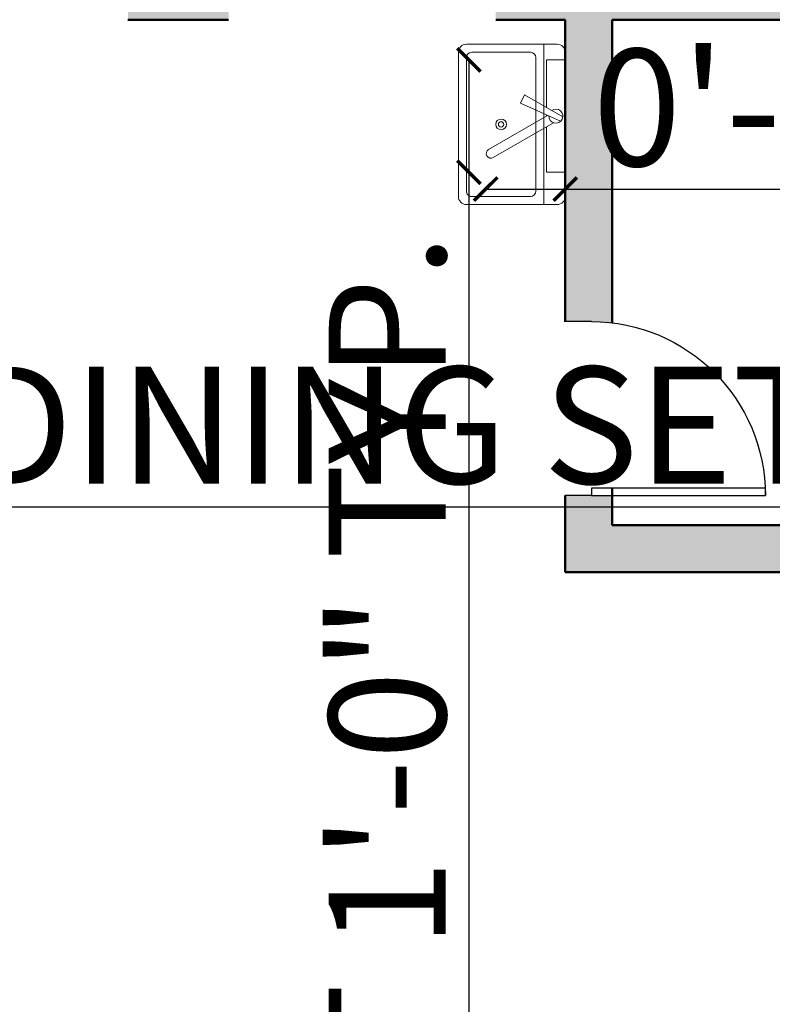
# Model space of a CAD drawing. Units: inches. Extents: x 2419 to 2878, y 1068 to 1713.
# Tile 11 of 20: x 2574 to 2655, y 1304 to 1409. Entities that reach past the tile are written whole.
import ezdxf

# ---------------------------------------------------------------- set-up
doc = ezdxf.new("R2010")
doc.units = ezdxf.units.IN
for name, color, linetype, lineweight in [('A-ANNO-DIMS', 2, 'Continuous', 18), ('A-DOOR', 4, 'Continuous', 25), ('A-FLOR-FIXT', 8, 'Continuous', 18), ('A-FLOR-PRKG-PATT', 1, 'Continuous', 13), ('A-WALL', 7, 'Continuous', 50)]:
    doc.layers.add(name, color=color, linetype=linetype, lineweight=lineweight)
doc.layers.add('A-WALL-PATT', color=18, linetype='Continuous', lineweight=13, true_color=0x000000)
doc.styles.get("Standard").update_dxf_attribs({"font": 'arial.ttf'})
doc.dimstyles.new('ISO-25', dxfattribs={"dimtxt": 12.5, "dimasz": 2.5, "dimexe": 1.25, "dimexo": 0.625, "dimtad": 1, "dimdec": 0, "dimlunit": 4, "dimtxsty": 'Standard', "dimblk": 'ARCHTICK', "dimcen": 2.5, "dimse1": 1, "dimse2": 1, "dimclrd": 4, "dimadec": 0, "dimazin": 0, "dimtfac": 1, "dimtdec": 0, "dimtmove": 0, "dimatfit": 3, "dimfxl": 1, "dimarcsym": 0})

# ---------------------------------------------------------------- blocks, each defined once
blk = doc.blocks.new('*U3')
for p, q in [((0, 0), (0, -6)), ((40, 0), (40, -6))]:
    blk.add_line(p, q)
blk.add_lwpolyline([(0, 0), (0, 40), (1.75, 40), (1.75, 0)], close=True)
blk.add_arc((0, 0), 40, 0, 90)
blk = doc.blocks.new('Sink-single - 30 in top')
blk.add_line((-15, -3.999996), (15, -3.999996))
for points in [[(-13.5, 0), (13.5, 0)], [(-15, -18.499996), (-15, -1.5)], [(15, -1.5), (15, -18.499996)], [(-12.5, -5.499996), (12.5, -5.499996)], [(-13.5, -17.499996), (-13.5, -6.499996)], [(13.5, -6.499996), (13.5, -17.499996)], [(13.5, -19.999996), (-13.5, -19.999996)], [(12.5, -18.499996), (-12.5, -18.499996)]]:
    blk.add_lwpolyline(points)
for radius in [1, 0.5]:
    blk.add_circle((0, -11.999996), radius)
for centre, radius, start, end in [((-13.5, -1.5), 1.5, 90, 180), ((13.5, -1.5), 1.5, 0, 90), ((-12.5, -6.499996), 1, 90, 180), ((12.5, -6.499996), 1, 0, 90), ((-12.5, -17.499996), 1, 180, 270), ((12.5, -17.499996), 1, 270, 0), ((-13.5, -18.499996), 1.5, 180, 270), ((13.5, -18.499996), 1.5, 270, 0)]:
    blk.add_arc(centre, radius, start, end)
blk = doc.blocks.new('Faucet - single handle top')
for p, q in [((0.08, -0.26), (-2.26, -4.34)), ((-1.37, -4.79), (0.55, -0.5)), ((-0.06, -1.9), (3.57, -8.18)), ((4.43, -7.68), (0.72, -1.24)), ((-2.26, -4.34), (-1.37, -4.79))]:
    blk.add_line(p, q)
for points in [[(-0.92, -2), (-6, -2), (-6, 0), (6, 0), (6, -2), (1.16, -2)], [(-0.01, -2), (-0.12, -2)]]:
    blk.add_lwpolyline(points)
for centre, radius, start, end in [((0, -1), 0.75, 269.2246, 216.2304), ((4, -7.93), 0.5, 210, 30)]:
    blk.add_arc(centre, radius, start, end)
blk = doc.blocks.new('_ArchTick')
at = {"color": 0, "linetype": 'ByBlock', "const_width": 0.15}
blk.add_lwpolyline([(-0.5, -0.5), (0.5, 0.5)], dxfattribs=at)
blk = doc.blocks.new('*D20')
at = {"layer": 'A-ANNO-DIMS', "color": 4, "lineweight": -2, "transparency": 16777216}
for p, q in [((2622.22, 1404.52), (2622.22, 1392.52)), ((2622.22, 1392.52), (2622.22, 1238.58))]:
    blk.add_line(p, q, dxfattribs=at)
at = {"layer": 'Defpoints', "color": 0, "transparency": 16777216}
for p in [(2624.02, 1404.52), (2622.22, 1392.52), (2624.02, 1392.52)]:
    blk.add_point(p, dxfattribs=at)
at = {"layer": 'A-ANNO-DIMS', "color": 4, "lineweight": -2, "transparency": 16777216, "xscale": 2.5, "yscale": 2.5, "zscale": 2.5}
for p, rotation in [((2622.22, 1404.52), 90), ((2622.22, 1392.52), 270)]:
    blk.add_blockref('_ArchTick', p, dxfattribs=dict(at, rotation=rotation))
at = {"layer": 'A-ANNO-DIMS', "color": 0, "transparency": 16777216, "insert": (2615.13, 1314.3), "char_height": 12.5, "attachment_point": 5, "rotation": 90}
blk.add_mtext('FAUCET 1\'-0" TYP.', dxfattribs=at)
blk = doc.blocks.new('*D21')
at = {"layer": 'A-ANNO-DIMS', "color": 4, "lineweight": -2, "transparency": 16777216}
for p, q in [((2624.02, 1390.72), (2632.51, 1390.72)), ((2632.51, 1390.72), (2741.59, 1390.72))]:
    blk.add_line(p, q, dxfattribs=at)
at = {"layer": 'Defpoints', "color": 0, "transparency": 16777216}
for p in [(2624.02, 1392.52), (2632.51, 1392.52), (2632.51, 1390.72)]:
    blk.add_point(p, dxfattribs=at)
at = {"layer": 'A-ANNO-DIMS', "color": 4, "lineweight": -2, "transparency": 16777216, "xscale": 2.5, "yscale": 2.5, "zscale": 2.5, "rotation": 180}
blk.add_blockref('_ArchTick', (2624.02, 1390.72), dxfattribs=at)
at = {"layer": 'A-ANNO-DIMS', "color": 4, "lineweight": -2, "transparency": 16777216, "xscale": 2.5, "yscale": 2.5, "zscale": 2.5}
blk.add_blockref('_ArchTick', (2632.51, 1390.72), dxfattribs=at)
at = {"layer": 'A-ANNO-DIMS', "color": 0, "transparency": 16777216, "insert": (2688.3, 1397.81), "char_height": 12.5, "attachment_point": 5}
blk.add_mtext('0\'-8 1/2" TYP.', dxfattribs=at)
blk = doc.blocks.new('*D26')
at = {"layer": 'A-ANNO-DIMS', "color": 4, "lineweight": -2, "transparency": 16777216}
for p, q in [((2502.77, 1356.79), (2563.46, 1356.79)), ((2563.46, 1356.79), (2733.72, 1356.79))]:
    blk.add_line(p, q, dxfattribs=at)
at = {"layer": 'Defpoints', "color": 0, "transparency": 16777216}
for p in [(2563.46, 1356.79), (2502.77, 1347.69), (2563.46, 1347.69)]:
    blk.add_point(p, dxfattribs=at)
at = {"layer": 'A-ANNO-DIMS', "color": 4, "lineweight": -2, "transparency": 16777216, "xscale": 2.5, "yscale": 2.5, "zscale": 2.5, "rotation": 180}
blk.add_blockref('_ArchTick', (2502.77, 1356.79), dxfattribs=at)
at = {"layer": 'A-ANNO-DIMS', "color": 4, "lineweight": -2, "transparency": 16777216, "xscale": 2.5, "yscale": 2.5, "zscale": 2.5}
blk.add_blockref('_ArchTick', (2563.46, 1356.79), dxfattribs=at)
at = {"layer": 'A-ANNO-DIMS', "color": 0, "transparency": 16777216, "insert": (2649.84, 1363.88), "char_height": 12.5, "attachment_point": 5}
blk.add_mtext('DINING SET 5\'-0 1/2"', dxfattribs=at)
blk = doc.blocks.new('*D44')
at = {"layer": 'A-ANNO-DIMS', "color": 4, "lineweight": -2, "transparency": 16777216}
for p, q in [((2557.3, 1079.92), (2585.82, 1079.92)), ((2585.82, 1079.92), (2652.14, 1079.92))]:
    blk.add_line(p, q, dxfattribs=at)
at = {"layer": 'Defpoints', "color": 0, "transparency": 16777216}
for p in [(2557.3, 1408.81), (2585.82, 1408.81), (2585.82, 1079.92)]:
    blk.add_point(p, dxfattribs=at)
at = {"layer": 'A-ANNO-DIMS', "color": 4, "lineweight": -2, "transparency": 16777216, "xscale": 2.5, "yscale": 2.5, "zscale": 2.5, "rotation": 180}
blk.add_blockref('_ArchTick', (2557.3, 1079.92), dxfattribs=at)
at = {"layer": 'A-ANNO-DIMS', "color": 4, "lineweight": -2, "transparency": 16777216, "xscale": 2.5, "yscale": 2.5, "zscale": 2.5}
blk.add_blockref('_ArchTick', (2585.82, 1079.92), dxfattribs=at)
at = {"layer": 'A-ANNO-DIMS', "color": 0, "transparency": 16777216, "insert": (2620.23, 1087.01), "char_height": 12.5, "attachment_point": 5}
blk.add_mtext('2\'-4 1/2"', dxfattribs=at)
blk = doc.blocks.new('*D45')
at = {"layer": 'A-ANNO-DIMS', "color": 4, "lineweight": -2, "transparency": 16777216}
for p, q in [((2596.57, 1079.92), (2625.09, 1079.92)), ((2625.09, 1079.92), (2691.41, 1079.92))]:
    blk.add_line(p, q, dxfattribs=at)
at = {"layer": 'Defpoints', "color": 0, "transparency": 16777216}
for p in [(2596.57, 1408.81), (2625.09, 1408.81), (2625.09, 1079.92)]:
    blk.add_point(p, dxfattribs=at)
at = {"layer": 'A-ANNO-DIMS', "color": 4, "lineweight": -2, "transparency": 16777216, "xscale": 2.5, "yscale": 2.5, "zscale": 2.5, "rotation": 180}
blk.add_blockref('_ArchTick', (2596.57, 1079.92), dxfattribs=at)
at = {"layer": 'A-ANNO-DIMS', "color": 4, "lineweight": -2, "transparency": 16777216, "xscale": 2.5, "yscale": 2.5, "zscale": 2.5}
blk.add_blockref('_ArchTick', (2625.09, 1079.92), dxfattribs=at)
at = {"layer": 'A-ANNO-DIMS', "color": 0, "transparency": 16777216, "insert": (2659.5, 1087.01), "char_height": 12.5, "attachment_point": 5}
blk.add_mtext('2\'-4 1/2"', dxfattribs=at)
blk = doc.blocks.new('*D47')
at = {"layer": 'A-ANNO-DIMS', "color": 4, "lineweight": -2, "transparency": 16777216}
for p, q in [((2444.31, 1376.56), (2444.31, 1357.98)), ((2444.31, 1357.98), (2444.31, 1293.05))]:
    blk.add_line(p, q, dxfattribs=at)
at = {"layer": 'Defpoints', "color": 0, "transparency": 16777216}
for p in [(2632.51, 1376.56), (2444.31, 1357.98), (2632.51, 1357.98)]:
    blk.add_point(p, dxfattribs=at)
at = {"layer": 'A-ANNO-DIMS', "color": 4, "lineweight": -2, "transparency": 16777216, "xscale": 2.5, "yscale": 2.5, "zscale": 2.5}
for p, rotation in [((2444.31, 1376.56), 90), ((2444.31, 1357.98), 270)]:
    blk.add_blockref('_ArchTick', p, dxfattribs=dict(at, rotation=rotation))
at = {"layer": 'A-ANNO-DIMS', "color": 0, "transparency": 16777216, "insert": (2437.23, 1324.26), "char_height": 12.5, "attachment_point": 5, "rotation": 90}
blk.add_mtext('1\'-6 1/2"', dxfattribs=at)
blk = doc.blocks.new('*D53')
at = {"layer": 'A-ANNO-DIMS', "color": 4, "lineweight": -2, "transparency": 16777216}
for p, q in [((2638.79, 1605.01), (2667.31, 1605.01)), ((2667.31, 1605.01), (2733.63, 1605.01))]:
    blk.add_line(p, q, dxfattribs=at)
at = {"layer": 'Defpoints', "color": 0, "transparency": 16777216}
for p in [(2667.31, 1605.01), (2638.79, 1217.38), (2667.31, 1217.38)]:
    blk.add_point(p, dxfattribs=at)
at = {"layer": 'A-ANNO-DIMS', "color": 4, "lineweight": -2, "transparency": 16777216, "xscale": 2.5, "yscale": 2.5, "zscale": 2.5, "rotation": 180}
blk.add_blockref('_ArchTick', (2638.79, 1605.01), dxfattribs=at)
at = {"layer": 'A-ANNO-DIMS', "color": 4, "lineweight": -2, "transparency": 16777216, "xscale": 2.5, "yscale": 2.5, "zscale": 2.5}
blk.add_blockref('_ArchTick', (2667.31, 1605.01), dxfattribs=at)
at = {"layer": 'A-ANNO-DIMS', "color": 0, "transparency": 16777216, "insert": (2701.72, 1612.1), "char_height": 12.5, "attachment_point": 5}
blk.add_mtext('2\'-4 1/2"', dxfattribs=at)
blk = doc.blocks.new('*D56')
at = {"layer": 'A-ANNO-DIMS', "color": 4, "lineweight": -2, "transparency": 16777216}
for p, q in [((2480.51, 1079.92), (2503.97, 1079.92)), ((2503.97, 1079.92), (2578.61, 1079.92))]:
    blk.add_line(p, q, dxfattribs=at)
at = {"layer": 'Defpoints', "color": 0, "transparency": 16777216}
for p in [(2480.51, 1507.81), (2503.97, 1494.85), (2503.97, 1079.92)]:
    blk.add_point(p, dxfattribs=at)
at = {"layer": 'A-ANNO-DIMS', "color": 4, "lineweight": -2, "transparency": 16777216, "xscale": 2.5, "yscale": 2.5, "zscale": 2.5, "rotation": 180}
blk.add_blockref('_ArchTick', (2480.51, 1079.92), dxfattribs=at)
at = {"layer": 'A-ANNO-DIMS', "color": 4, "lineweight": -2, "transparency": 16777216, "xscale": 2.5, "yscale": 2.5, "zscale": 2.5}
blk.add_blockref('_ArchTick', (2503.97, 1079.92), dxfattribs=at)
at = {"layer": 'A-ANNO-DIMS', "color": 0, "transparency": 16777216, "insert": (2542.54, 1087.01), "char_height": 12.5, "attachment_point": 5}
blk.add_mtext('1\'-11 1/2"', dxfattribs=at)
blk = doc.blocks.new('*D59')
at = {"layer": 'A-ANNO-DIMS', "color": 4, "lineweight": -2, "transparency": 16777216}
blk.add_line((2480.51, 1079.92), (2589.51, 1079.92), dxfattribs=at)
at = {"layer": 'Defpoints', "color": 0, "transparency": 16777216}
for p in [(2480.51, 1414.81), (2589.51, 1414.81), (2589.51, 1079.92)]:
    blk.add_point(p, dxfattribs=at)
at = {"layer": 'A-ANNO-DIMS', "color": 4, "lineweight": -2, "transparency": 16777216, "xscale": 2.5, "yscale": 2.5, "zscale": 2.5, "rotation": 180}
blk.add_blockref('_ArchTick', (2480.51, 1079.92), dxfattribs=at)
at = {"layer": 'A-ANNO-DIMS', "color": 4, "lineweight": -2, "transparency": 16777216, "xscale": 2.5, "yscale": 2.5, "zscale": 2.5}
blk.add_blockref('_ArchTick', (2589.51, 1079.92), dxfattribs=at)
at = {"layer": 'A-ANNO-DIMS', "color": 0, "transparency": 16777216, "insert": (2535.01, 1086.93), "char_height": 12.5, "attachment_point": 5}
blk.add_mtext('9\'-1"', dxfattribs=at)

msp = doc.modelspace()

# ---------------------------------------------------------------- hatches: boundary and pattern name
at = {"layer": 'A-FLOR-PRKG-PATT'}
h = msp.add_hatch(color=256, dxfattribs=at)
h.dxf.hatch_style = 1
edge = h.paths.add_edge_path()
edge.add_ellipse((2561.37, 1279.45), major_axis=(3.99, 0), ratio=0.842304, start_angle=0.6466, end_angle=90)
edge.add_line((2561.37, 1282.81), (2511.57, 1282.81))
edge.add_ellipse((2511.57, 1279.45), major_axis=(3.99, 0), ratio=0.842304, start_angle=90, end_angle=179.3534)
edge.add_ellipse((10560.89, 1188.62), major_axis=(-8054.03, 0), ratio=0.8423039, start_angle=-0.646554, end_angle=-0.628237)
edge.add_ellipse((2509.23, 1276.91), major_axis=(1.69, 0), ratio=0.842304, start_angle=179.3718, end_angle=248.4648)
edge.add_ellipse((10560.33, 1188.62), major_axis=(8052.29, 0), ratio=0.8423039, start_angle=179.353446, end_angle=179.381357, ccw=False)
edge.add_ellipse((2511.01, 1279.45), major_axis=(2.25, 0), ratio=0.842304, start_angle=90, end_angle=179.3534, ccw=False)
edge.add_line((2511.01, 1281.35), (2561.94, 1281.35))
edge.add_ellipse((2561.94, 1279.45), major_axis=(-2.25, 0), ratio=0.842304, start_angle=180.6466, end_angle=270, ccw=False)
edge.add_ellipse((-5487.38, 1188.62), major_axis=(8052.29, 0), ratio=0.8423039, start_angle=0.528271, end_angle=0.646554, ccw=False)
edge.add_ellipse((2563.71, 1276.91), major_axis=(-1.69, 0), ratio=0.842304, start_angle=111.5352, end_angle=180.6282)
edge.add_ellipse((-5487.95, 1188.62), major_axis=(-8054.03, 0), ratio=0.8423039, start_angle=180.628237, end_angle=180.646554)
edge = h.paths.add_edge_path()
edge.add_ellipse((2564.91, 1261.91), major_axis=(-1.12, 0), ratio=0.842304, start_angle=180, end_angle=270)
edge.add_line((2564.91, 1262.86), (2564.43, 1262.86))
edge.add_ellipse((-5487.38, 1188.62), major_axis=(8052.29, 0), ratio=0.8423039, start_angle=0.383867, end_angle=0.528271, ccw=False)
edge.add_line((2564.65, 1242.56), (2564.91, 1242.56))
edge.add_ellipse((2564.91, 1243.51), major_axis=(-1.12, 0), ratio=0.842304, start_angle=90, end_angle=180)
edge.add_line((2566.03, 1243.51), (2566.03, 1261.91))
edge = h.paths.add_edge_path()
edge.add_ellipse((2564.91, 1174.99), major_axis=(1.12, 0), ratio=0.842304, start_angle=0, end_angle=90)
edge.add_line((2564.91, 1175.94), (2564.89, 1175.94))
edge.add_ellipse((-5487.38, 1188.62), major_axis=(8052.29, 0), ratio=0.8423039, start_angle=-0.134987, end_angle=-0.090229, ccw=False)
edge.add_ellipse((2163.34, 1170.91), major_axis=(401.54, 0), ratio=0.842304, start_angle=-2.18, end_angle=-0.1356, ccw=False)
edge.add_line((2564.47, 1155.64), (2564.91, 1155.64))
edge.add_ellipse((2564.91, 1156.59), major_axis=(-1.12, 0), ratio=0.842304, start_angle=90, end_angle=180)
edge.add_line((2566.03, 1156.59), (2566.03, 1174.99))
h.paths.add_polyline_path([(2574.48, 1207.45), (2633.94, 1207.45), (2633.94, 1217.37), (2574.48, 1217.37)], flags=9)
h.paths.add_polyline_path([(2574.45, 1217.83), (2610.47, 1217.83), (2610.47, 1227.88), (2574.45, 1227.88)], flags=9)
h.paths.add_polyline_path([(2672.43, 1304.02), (2718.62, 1304.02), (2718.62, 1313.94), (2672.43, 1313.94)], flags=9)
h.paths.add_polyline_path([(2672.4, 1314.4), (2750.13, 1314.4), (2750.13, 1324.45), (2672.4, 1324.45)], flags=9)
h.paths.add_polyline_path([(2500.43, 1374.44), (2544.8, 1374.44), (2544.8, 1384.36), (2500.43, 1384.36)], flags=9)
h.paths.add_polyline_path([(2500.41, 1384.82), (2566.08, 1384.82), (2566.08, 1394.87), (2500.41, 1394.87)], flags=9)
h.paths.add_polyline_path([(2738.93, 1376.75), (2778.27, 1376.75), (2778.27, 1386.67), (2738.93, 1386.67)], flags=9)
h.paths.add_polyline_path([(2659.12, 1357.8), (2703.49, 1357.8), (2703.49, 1367.72), (2659.12, 1367.72)], flags=9)
h.paths.add_polyline_path([(2659.1, 1368.18), (2694.11, 1368.18), (2694.11, 1378.23), (2659.1, 1378.23)], flags=9)
h.paths.add_polyline_path([(2730.12, 1466.07), (2769.46, 1466.07), (2769.46, 1475.99), (2730.12, 1475.99)], flags=9)
h.paths.add_polyline_path([(2730.1, 1476.45), (2765.12, 1476.45), (2765.12, 1486.5), (2730.1, 1486.5)], flags=9)
h.paths.add_polyline_path([(2730.38, 1518.65), (2761.48, 1518.65), (2761.48, 1528.57), (2730.38, 1528.57)], flags=9)
h.paths.add_polyline_path([(2730.36, 1529.03), (2780.96, 1529.03), (2780.96, 1539.07), (2730.36, 1539.07)], flags=9)
h.paths.add_polyline_path([(2629.32, 1455.19), (2688.78, 1455.19), (2688.78, 1465.11), (2629.32, 1465.11)], flags=9)
h.paths.add_polyline_path([(2629.3, 1465.57), (2681.9, 1465.57), (2681.9, 1475.62), (2629.3, 1475.62)], flags=9)
h.paths.add_polyline_path([(2513.23, 1456.48), (2562.63, 1456.48), (2562.63, 1466.4), (2513.23, 1466.4)], flags=9)
h.paths.add_polyline_path([(2513.21, 1466.86), (2556.26, 1466.86), (2556.26, 1476.91), (2513.21, 1476.91)], flags=9)
h.paths.add_polyline_path([(2488.87, 1521.54), (2519.97, 1521.54), (2519.97, 1531.46), (2488.87, 1531.46)], flags=9)
h.paths.add_polyline_path([(2536.55, 1543.51), (2580.92, 1543.51), (2580.92, 1553.43), (2536.55, 1553.43)], flags=9)
h.paths.add_polyline_path([(2536.56, 1553.92), (2573.53, 1553.92), (2573.53, 1563.8), (2536.56, 1563.8)], flags=9)
at = {"layer": 'A-WALL-PATT'}
h = msp.add_hatch(color=256, dxfattribs=at)
h.dxf.hatch_style = 1
h.paths.add_polyline_path([(2780.51, 1577.81), (2471.51, 1577.81), (2471.51, 1121.81), (2780.51, 1121.81)])
h.paths.add_polyline_path([(2480.51, 1568.81), (2771.51, 1568.81), (2771.51, 1130.81), (2480.51, 1130.81)], flags=16)
h.paths.add_polyline_path([(2528.51, 1568.81), (2528.51, 1512.81), (2594.51, 1512.81), (2594.51, 1414.81), (2596.57, 1414.81), (2596.57, 1441.61), (2597.82, 1441.61), (2597.82, 1441.58, -0.384016), (2625.03, 1414.81), (2725.51, 1414.81), (2725.51, 1567.55), (2728.3, 1567.55), (2746.89, 1567.55), (2746.89, 1566.73), (2746.87, 1566.73, -0.367216), (2730.51, 1549.09), (2730.51, 1512.81), (2750.85, 1512.81), (2750.85, 1510.03, -0.401453), (2733.08, 1491.46), (2733.08, 1491.44), (2732.27, 1491.44), (2732.27, 1507.81), (2730.51, 1507.81), (2730.51, 1408.81), (2736.51, 1408.81), (2736.51, 1349.81), (2632.51, 1349.81), (2632.51, 1408.81), (2528.51, 1408.81), (2528.51, 1414.81), (2503.97, 1414.81), (2503.97, 1494.85), (2558.38, 1494.85), (2558.38, 1507.81), (2529.96, 1507.81, -0.414214), (2530.82, 1506.96), (2530.82, 1497.26, -0.414214), (2529.96, 1496.4), (2514.56, 1496.4, -0.414214), (2513.7, 1497.26), (2513.7, 1506.96, -0.414214), (2514.56, 1507.81), (2528.51, 1507.81), (2528.51, 1512.81), (2480.51, 1512.81)], flags=0)
h.paths.add_polyline_path([(2516.26, 1507.81), (2528.26, 1507.81), (2528.26, 1505.81), (2523.42, 1505.81), (2524.07, 1504.67), (2529.39, 1504.67, -0.414214), (2529.96, 1504.1), (2529.96, 1497.83, -0.414214), (2529.39, 1497.26), (2515.13, 1497.26, -0.414214), (2514.56, 1497.83), (2514.56, 1504.1, -0.414214), (2515.13, 1504.67), (2520.69, 1504.67), (2521.34, 1505.81), (2516.26, 1505.81)], flags=0)
h.paths.add_polyline_path([(2522.02, 1505.53), (2522.82, 1507.32, -0.65506), (2522.25, 1506.06), (2522.19, 1505.93), (2522.43, 1505.53)], flags=0)
h.paths.add_polyline_path([(2522.83, 1500.97, -1), (2521.69, 1500.97, -1)], flags=0)
h.paths.add_polyline_path([(2522.55, 1500.97, -1), (2521.98, 1500.97, -1)], flags=0)
h.paths.add_polyline_path([(2482.01, 1470.63), (2499.89, 1470.63), (2499.89, 1448.27), (2482.01, 1448.27), (2482.01, 1452.74), (2481.26, 1452.74), (2481.26, 1449.76), (2480.51, 1449.76), (2480.51, 1469.14), (2481.26, 1469.14), (2481.26, 1466.16), (2482.01, 1466.16)], flags=0)
h.paths.add_polyline_path([(2488.71, 1466.16, -1), (2484.24, 1466.16, -1)], flags=0)
h.paths.add_polyline_path([(2496.17, 1466.16, -1), (2490.2, 1466.16, -1)], flags=0)
h.paths.add_polyline_path([(2487.97, 1466.16, -1), (2484.99, 1466.16, -1)], flags=0)
h.paths.add_polyline_path([(2495.42, 1466.16, -1), (2490.95, 1466.16, -1)], flags=0)
h.paths.add_polyline_path([(2487.22, 1466.16, -1), (2485.73, 1466.16, -1)], flags=0)
h.paths.add_polyline_path([(2494.68, 1466.16, -1), (2491.69, 1466.16, -1)], flags=0)
h.paths.add_polyline_path([(2499.11, 1468, -1), (2497.98, 1468, -1)], flags=0)
h.paths.add_polyline_path([(2493.93, 1466.16, -1), (2492.44, 1466.16, -1)], flags=0)
h.paths.add_polyline_path([(2499.37, 1463.71, -1), (2498.17, 1463.71, -1)], flags=0)
h.paths.add_polyline_path([(2484.24, 1461.69), (2496.17, 1461.69), (2496.17, 1457.22), (2484.24, 1457.22)], flags=0)
h.paths.add_polyline_path([(2484.99, 1460.94), (2495.42, 1460.94), (2495.42, 1457.96), (2484.99, 1457.96)], flags=0)
h.paths.add_polyline_path([(2586.88, 1510.03), (2587.69, 1510.03), (2587.69, 1491.44), (2586.88, 1491.44)], flags=0)
h.paths.add_polyline_path([(2499.26, 1459.41, -1), (2498.2, 1459.41, -1)], flags=0)
h.paths.add_polyline_path([(2489.46, 1452.74, -1), (2483.5, 1452.74, -1)], flags=0)
h.paths.add_polyline_path([(2557.3, 1408.81), (2557.3, 1413.09, -0.401453), (2584.57, 1441.58), (2584.57, 1441.61), (2585.82, 1441.61), (2585.82, 1413.09), (2585.82, 1408.81)], flags=0)
h.paths.add_polyline_path([(2488.71, 1452.74, -1), (2484.24, 1452.74, -1)], flags=0)
h.paths.add_polyline_path([(2495.42, 1452.74, -1), (2490.95, 1452.74, -1)], flags=0)
h.paths.add_polyline_path([(2487.97, 1452.74, -1), (2484.99, 1452.74, -1)], flags=0)
h.paths.add_polyline_path([(2494.68, 1452.74, -1), (2491.69, 1452.74, -1)], flags=0)
h.paths.add_polyline_path([(2487.22, 1452.74, -1), (2485.73, 1452.74, -1)], flags=0)
h.paths.add_polyline_path([(2499.18, 1454.44, -1), (2497.9, 1454.44, -1)], flags=0)
h.paths.add_polyline_path([(2493.93, 1452.74, -1), (2492.44, 1452.74, -1)], flags=0)
h.paths.add_polyline_path([(2499.3, 1450.64, -1), (2497.79, 1450.64, -1)], flags=0)
h.paths.add_polyline_path([(2619.13, 1558.89, -1), (2605.13, 1558.89, -1)], flags=0)
h.paths.add_polyline_path([(2609.13, 1558.89), (2612.13, 1561.89), (2615.13, 1558.89), (2612.13, 1555.89)], flags=0)
h.paths.add_polyline_path([(2611.13, 1558.89, -1), (2613.13, 1558.89, -1)], flags=0)
h.paths.add_polyline_path([(2633.68, 1568.81), (2693.68, 1568.81), (2693.68, 1488.81), (2633.68, 1488.81)], flags=0)
h.paths.add_polyline_path([(2641.68, 1554.41), (2641.68, 1567.61), (2662.48, 1567.61), (2662.48, 1554.41), (2664.88, 1554.41), (2664.88, 1567.61), (2685.68, 1567.61), (2685.68, 1552.41), (2680.48, 1552.41), (2693.68, 1539.21), (2678.48, 1539.21), (2678.48, 1554.41)], flags=0)
h.paths.add_polyline_path([(2637.51, 1408.81), (2731.51, 1408.81), (2731.51, 1354.81), (2637.51, 1354.81), (2637.51, 1357.98), (2635.3, 1357.98), (2635.3, 1358.79), (2637.51, 1358.79)], flags=0)
h.paths.add_polyline_path([(2717.17, 1559.64, -1), (2703.17, 1559.64, -1)], flags=0)
h.paths.add_polyline_path([(2707.17, 1559.64), (2710.17, 1562.64), (2713.17, 1559.64), (2710.17, 1556.64)], flags=0)
h.paths.add_polyline_path([(2709.17, 1559.64, -1), (2711.17, 1559.64, -1)], flags=0)
h.paths.add_polyline_path([(2685.38, 1408.81), (2706.38, 1408.81), (2706.38, 1400.81), (2699.88, 1400.81), (2701.88, 1394.81, -0.501323), (2696.92, 1375.95, -0.132891), (2694.83, 1375.95, -0.501317), (2689.88, 1394.81), (2691.88, 1400.81), (2688.88, 1400.81), (2688.88, 1399.31), (2685.88, 1399.31), (2685.88, 1400.31), (2687.88, 1400.31), (2687.88, 1400.81), (2685.38, 1400.81)], flags=0)
h.paths.add_polyline_path([(2687.38, 1407.81), (2704.38, 1407.81, -0.5), (2705.38, 1406.81), (2705.38, 1402.81, -0.5), (2704.38, 1401.81), (2687.38, 1401.81, -0.5), (2686.38, 1402.81), (2686.38, 1406.81, -0.5)], flags=0)
h.paths.add_polyline_path([(2639.51, 1205.81), (2634.51, 1205.81), (2634.51, 1293.81), (2637.51, 1293.81), (2639.51, 1293.81)], flags=0)
h.paths.add_polyline_path([(2691.88, 1394.81), (2699.88, 1394.81, -0.48008), (2697.52, 1377.29, -0.215004), (2694.23, 1377.29, -0.48008)], flags=0)
h.paths.add_polyline_path([(2757.51, 1453.89), (2763.51, 1451.89), (2763.51, 1454.89), (2762.01, 1454.89), (2762.01, 1457.89), (2763.01, 1457.89), (2763.01, 1455.89), (2763.51, 1455.89), (2763.51, 1458.39), (2771.51, 1458.39), (2771.51, 1437.39), (2763.51, 1437.39), (2763.51, 1443.89), (2757.51, 1441.89, -0.501323), (2738.65, 1446.85, -0.132891), (2738.65, 1448.94, -0.501317)], flags=0)
h.paths.add_polyline_path([(2739.99, 1449.54, -0.48008), (2757.51, 1451.89), (2757.51, 1443.89, -0.48008), (2739.99, 1446.25, -0.215004)], flags=0)
h.paths.add_polyline_path([(2765.51, 1457.39), (2769.51, 1457.39, -0.5), (2770.51, 1456.39), (2770.51, 1439.39, -0.5), (2769.51, 1438.39), (2765.51, 1438.39, -0.5), (2764.51, 1439.39), (2764.51, 1456.39, -0.5)], flags=0)
h = msp.add_hatch(color=256, dxfattribs=at)
h.dxf.hatch_style = 1
h.paths.add_polyline_path([(2771.51, 1354.81), (2736.51, 1354.81), (2736.51, 1408.81), (2771.51, 1408.81), (2771.51, 1414.81), (2625.03, 1414.81, -0.015108), (2625.09, 1413.09), (2625.09, 1408.81), (2632.51, 1408.81), (2632.51, 1376.56), (2635.3, 1376.56, -0.029838), (2637.51, 1376.43), (2637.51, 1408.81), (2731.51, 1408.81), (2731.51, 1354.81), (2637.51, 1354.81), (2637.51, 1357.98), (2635.3, 1357.98), (2632.51, 1357.98), (2632.51, 1349.81), (2771.51, 1349.81)])
h.paths.add_polyline_path([(2639.51, 1298.81), (2637.51, 1298.81), (2480.51, 1298.81), (2480.51, 1293.81), (2637.51, 1293.81), (2639.51, 1293.81)])
h.paths.add_polyline_path([(2639.51, 1293.81), (2637.51, 1293.81), (2634.51, 1293.81), (2634.51, 1244.65), (2638.79, 1244.65, -0.006332), (2639.51, 1244.64)])
h.paths.add_polyline_path([(2639.51, 1205.81), (2771.51, 1205.81), (2771.51, 1210.81), (2639.51, 1210.81), (2639.51, 1216.13), (2638.79, 1216.13), (2634.51, 1216.13), (2634.51, 1130.81), (2639.51, 1130.81)])
h.paths.add_polyline_path([(2596.57, 1413.09), (2596.57, 1414.81), (2585.82, 1414.81), (2585.82, 1413.09), (2585.82, 1408.81), (2596.57, 1408.81)])
h.paths.add_polyline_path([(2557.3, 1413.09, -0.015108), (2557.35, 1414.81), (2480.51, 1414.81), (2480.51, 1408.81), (2557.3, 1408.81)])
h.paths.add_polyline_path([(2574.48, 1207.45), (2633.94, 1207.45), (2633.94, 1217.37), (2574.48, 1217.37)], flags=9)
h.paths.add_polyline_path([(2574.45, 1217.83), (2610.47, 1217.83), (2610.47, 1227.88), (2574.45, 1227.88)], flags=9)
h.paths.add_polyline_path([(2672.43, 1304.02), (2718.62, 1304.02), (2718.62, 1313.94), (2672.43, 1313.94)], flags=9)
h.paths.add_polyline_path([(2672.4, 1314.4), (2750.13, 1314.4), (2750.13, 1324.45), (2672.4, 1324.45)], flags=9)
h.paths.add_polyline_path([(2500.43, 1374.44), (2544.8, 1374.44), (2544.8, 1384.36), (2500.43, 1384.36)], flags=9)
h.paths.add_polyline_path([(2500.41, 1384.82), (2566.08, 1384.82), (2566.08, 1394.87), (2500.41, 1394.87)], flags=9)
h.paths.add_polyline_path([(2738.93, 1376.75), (2778.27, 1376.75), (2778.27, 1386.67), (2738.93, 1386.67)], flags=9)
h.paths.add_polyline_path([(2659.12, 1357.8), (2703.49, 1357.8), (2703.49, 1367.72), (2659.12, 1367.72)], flags=25)
h.paths.add_polyline_path([(2659.1, 1368.18), (2694.11, 1368.18), (2694.11, 1378.23), (2659.1, 1378.23)], flags=25)
h.paths.add_polyline_path([(2730.12, 1466.07), (2769.46, 1466.07), (2769.46, 1475.99), (2730.12, 1475.99)], flags=9)
h.paths.add_polyline_path([(2730.1, 1476.45), (2765.12, 1476.45), (2765.12, 1486.5), (2730.1, 1486.5)], flags=9)
h.paths.add_polyline_path([(2730.38, 1518.65), (2761.48, 1518.65), (2761.48, 1528.57), (2730.38, 1528.57)], flags=9)
h.paths.add_polyline_path([(2730.36, 1529.03), (2780.96, 1529.03), (2780.96, 1539.07), (2730.36, 1539.07)], flags=9)
h.paths.add_polyline_path([(2629.32, 1455.19), (2688.78, 1455.19), (2688.78, 1465.11), (2629.32, 1465.11)], flags=9)
h.paths.add_polyline_path([(2629.3, 1465.57), (2681.9, 1465.57), (2681.9, 1475.62), (2629.3, 1475.62)], flags=9)
h.paths.add_polyline_path([(2513.23, 1456.48), (2562.63, 1456.48), (2562.63, 1466.4), (2513.23, 1466.4)], flags=9)
h.paths.add_polyline_path([(2513.21, 1466.86), (2556.26, 1466.86), (2556.26, 1476.91), (2513.21, 1476.91)], flags=9)
h.paths.add_polyline_path([(2488.87, 1521.54), (2519.97, 1521.54), (2519.97, 1531.46), (2488.87, 1531.46)], flags=9)
h.paths.add_polyline_path([(2536.55, 1543.51), (2580.92, 1543.51), (2580.92, 1553.43), (2536.55, 1553.43)], flags=9)
h.paths.add_polyline_path([(2536.56, 1553.92), (2573.53, 1553.92), (2573.53, 1563.8), (2536.56, 1563.8)], flags=9)

# ---------------------------------------------------------------- linework, layer by layer
at = {"layer": 'A-WALL'}
for p, q in [((2585.82, 1408.81), (2596.57, 1408.81)), ((2585.82, 1408.81), (2596.57, 1408.81)), ((2625.09, 1408.81), (2632.51, 1408.81)), ((2625.09, 1408.81), (2632.51, 1408.81)), ((2632.51, 1376.56), (2632.51, 1408.81)), ((2637.51, 1408.81), (2637.51, 1376.43)), ((2637.51, 1408.81), (2731.51, 1408.81)), ((2637.51, 1408.81), (2731.51, 1408.81)), ((2637.51, 1358.79), (2637.51, 1354.81)), ((2632.51, 1349.81), (2632.51, 1357.98)), ((2637.51, 1354.81), (2731.51, 1354.81)), ((2632.51, 1349.81), (2771.51, 1349.81))]:
    msp.add_line(p, q, dxfattribs=at)

# ---------------------------------------------------------------- block references
at = {"layer": 'A-DOOR', "xscale": -0.4646269055216028, "yscale": 0.4646269055216028, "zscale": 0.4646269055216028, "rotation": 270}
msp.add_blockref('*U3', (2635.3, 1357.98), dxfattribs=at)
at = {"layer": 'A-FLOR-FIXT', "xscale": 0.5705899714795267, "yscale": 0.5705899714795267, "zscale": 0.5705899714795267, "rotation": 270}
msp.add_blockref('Sink-single - 30 in top', (2632.51, 1397.63), dxfattribs=at)
at = {"layer": 'A-FLOR-FIXT', "rotation": 270}
msp.add_blockref('Faucet - single handle top', (2632.51, 1398.52), dxfattribs=at)

# ---------------------------------------------------------------- dimensions: what is measured, and where the dimension line sits
at = {"layer": 'A-ANNO-DIMS'}
for base, p1, p2, picture, middle in [((2667.31, 1605.01), (2638.79, 1217.38), (2667.31, 1217.38), '*D53', (2701.72, 1612.1)), ((2503.97, 1079.92), (2480.51, 1507.81), (2503.97, 1494.85), '*D56', (2542.54, 1087.01)), ((2589.51, 1079.92), (2480.51, 1414.81), (2589.51, 1414.81), '*D59', (2535.01, 1086.93)), ((2585.82, 1079.92), (2557.3, 1408.81), (2585.82, 1408.81), '*D44', (2620.23, 1087.01)), ((2625.09, 1079.92), (2596.57, 1408.81), (2625.09, 1408.81), '*D45', (2659.5, 1087.01))]:
    dim = msp.add_linear_dim(base=base, p1=p1, p2=p2, dimstyle='ISO-25', override={"dimdec": 1, "dimlfac": 1, "dimrnd": 0, "dimzin": 1, "dimdsep": 46, "dimlunit": 4, "dimfrac": 2}, dxfattribs=at)
    dim.commit()
    dim.dimension.update_dxf_attribs({"geometry": picture, "text_midpoint": middle})
for base, p1, p2, text, picture, middle in [((2632.51, 1390.72), (2624.02, 1392.52), (2632.51, 1392.52), '<> TYP.', '*D21', (2688.3, 1397.81)), ((2563.46, 1356.79), (2502.77, 1347.69), (2563.46, 1347.69), 'DINING SET <>', '*D26', (2649.84, 1363.88))]:
    dim = msp.add_linear_dim(base=base, p1=p1, p2=p2, text=text, dimstyle='ISO-25', override={"dimdec": 1, "dimlfac": 1, "dimrnd": 0, "dimzin": 1, "dimdsep": 46, "dimlunit": 4, "dimfrac": 2}, dxfattribs=at)
    dim.commit()
    dim.dimension.update_dxf_attribs({"geometry": picture, "text_midpoint": middle})
dim = msp.add_linear_dim(base=(2622.22, 1392.52), p1=(2624.02, 1404.52), p2=(2624.02, 1392.52), angle=270, text='FAUCET <> TYP.', dimstyle='ISO-25', override={"dimdec": 1, "dimlfac": 1, "dimrnd": 0, "dimzin": 1, "dimdsep": 46, "dimlunit": 4, "dimfrac": 2}, dxfattribs=at)
dim.commit()
dim.dimension.update_dxf_attribs({"geometry": '*D20', "text_midpoint": (2615.13, 1314.3)})
dim = msp.add_linear_dim(base=(2444.31, 1357.98), p1=(2632.51, 1376.56), p2=(2632.51, 1357.98), angle=90, dimstyle='ISO-25', override={"dimdec": 1, "dimlfac": 1, "dimrnd": 0, "dimzin": 1, "dimdsep": 46, "dimlunit": 4, "dimfrac": 2}, dxfattribs=at)
dim.commit()
dim.dimension.update_dxf_attribs({"geometry": '*D47', "text_midpoint": (2437.23, 1324.26)})

doc.saveas('drawing.dxf')
